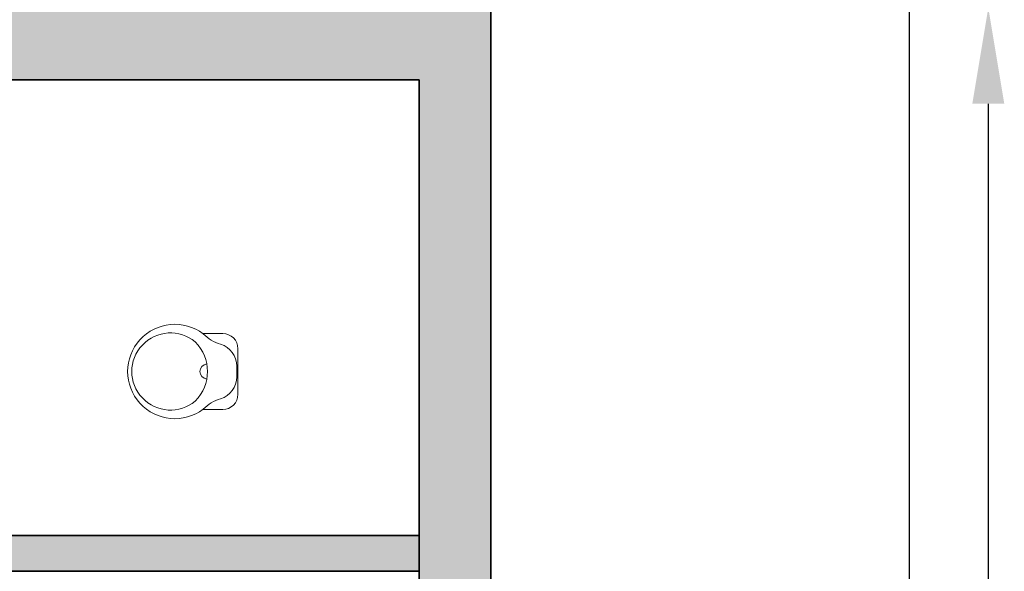
# Model space of a CAD drawing. Units: inches. Extents: x 2083 to 3317, y 1141 to 2115.
# Tile 249 of 256: x 3068 to 3191, y 1416 to 1485. Entities that reach past the tile are written whole.
import ezdxf

# ---------------------------------------------------------------- set-up
doc = ezdxf.new("R2010")
doc.units = ezdxf.units.IN
for name, color, linetype, lineweight in [('A-ANNO-DIMS', 2, 'Continuous', 18), ('A-FLOR-CASE', 8, 'Continuous', 18), ('A-FLOR-FIXT', 9, 'Continuous', 18), ('A-WALL', 7, 'Continuous', 35)]:
    doc.layers.add(name, color=color, linetype=linetype, lineweight=lineweight)
doc.layers.add('A-WALL-PATT', color=251, linetype='Continuous', lineweight=13, true_color=0x636466)
doc.styles.get("Standard").update_dxf_attribs({"font": 'arial.ttf'})
doc.dimstyles.new('ISO-25', dxfattribs={"dimtxt": 12, "dimasz": 12, "dimexe": 1.25, "dimexo": 0.625, "dimtad": 1, "dimlunit": 3, "dimtxsty": 'Standard', "dimcen": 2.5, "dimadec": 0, "dimazin": 0, "dimtfac": 1, "dimtmove": 0, "dimatfit": 3, "dimfxl": 1, "dimarcsym": 0})

# ---------------------------------------------------------------- blocks, each defined once
blk = doc.blocks.new('A$C6EF51710')
at = {"linetype": 'ByBlock'}
for p, q in [((0.0508, 0.2843), (0.1169, 0.2843)), ((0, 0.0811), (0, 0.2335)), ((0.0041, 0.1392), (0.0041, 0.1755)), ((0.1169, 0.0303), (0.0508, 0.0303))]:
    blk.add_line(p, q, dxfattribs=at)
for centre, radius, start, end in [((0.2107, 0.1573), 0.1576, 232.8984, 127.1016), ((0.0508, 0.2335), 0.0508, 90, 180), ((0.0168, 0.3818), 0.1397, 287.1046, 315), ((0.2254, 0.1573), 0.1289, 230.0084, 129.9916), ((0.0803, 0.1755), 0.0762, 107.1046, 180), ((0.2413, 0.1573), 0.1397, 135, 225), ((0.1016, 0.1573), 0.0254, 275.2159, 84.7841), ((0.0803, 0.1392), 0.0762, 180, 252.8954), ((0.0508, 0.0811), 0.0508, 180, 270), ((0.0168, -0.0672), 0.1397, 45, 72.8954)]:
    blk.add_arc(centre, radius, start, end, dxfattribs=at)
blk = doc.blocks.new('*D9')
at = {"layer": 'A-ANNO-DIMS', "color": 0, "lineweight": -2, "transparency": 16777216}
for p, q in [((3127.58, 1486.76), (3190.4, 1486.76)), ((3189.15, 1474.76), (3189.15, 1275.26)), ((3127.58, 1263.26), (3190.4, 1263.26))]:
    blk.add_line(p, q, dxfattribs=at)
at = {"layer": 'A-ANNO-DIMS', "color": 0, "transparency": 16777216}
for points in [[(3187.15, 1474.76), (3191.15, 1474.76), (3189.15, 1486.76)], [(3187.15, 1275.26), (3191.15, 1275.26), (3189.15, 1263.26)]]:
    blk.add_solid(points, dxfattribs=at)
at = {"layer": 'Defpoints', "color": 0, "transparency": 16777216}
for p in [(3126.96, 1486.76), (3126.96, 1263.26), (3189.15, 1263.26)]:
    blk.add_point(p, dxfattribs=at)
at = {"layer": 'A-ANNO-DIMS', "color": 0, "transparency": 16777216, "insert": (3182.4, 1375.01), "char_height": 12, "attachment_point": 5, "rotation": 90}
blk.add_mtext('18\'-7.5"', dxfattribs=at)
blk = doc.blocks.new('CASEWORK-96X24')
for q in [(0, 0), (24, 96)]:
    blk.add_line((0, 96), q)
blk = doc.blocks.new('*D35')
at = {"layer": 'A-ANNO-DIMS', "color": 0, "lineweight": -2, "transparency": 16777216}
for p, q in [((3127.58, 2020.76), (3180.56, 2020.76)), ((3179.31, 1275.26), (3179.31, 2008.76)), ((3127.58, 1263.26), (3180.56, 1263.26))]:
    blk.add_line(p, q, dxfattribs=at)
at = {"layer": 'A-ANNO-DIMS', "color": 0, "transparency": 16777216}
for points in [[(3177.31, 2008.76), (3181.31, 2008.76), (3179.31, 2020.76)], [(3177.31, 1275.26), (3181.31, 1275.26), (3179.31, 1263.26)]]:
    blk.add_solid(points, dxfattribs=at)
at = {"layer": 'Defpoints', "color": 0, "transparency": 16777216}
for p in [(3126.96, 2020.76), (3179.31, 2020.76), (3126.96, 1263.26)]:
    blk.add_point(p, dxfattribs=at)
at = {"layer": 'A-ANNO-DIMS', "color": 0, "transparency": 16777216, "insert": (3172.48, 1642.01), "char_height": 12, "attachment_point": 5, "rotation": 90}
blk.add_mtext('63\'-1 1/2"', dxfattribs=at)

msp = doc.modelspace()

# ---------------------------------------------------------------- hatches: boundary and pattern name
at = {"layer": 'A-WALL-PATT'}
h = msp.add_hatch(color=256, dxfattribs=at)
h.dxf.hatch_style = 1
h.paths.add_polyline_path([(3126.96, 2020.761), (2748.96, 2020.761), (2604.96, 2020.761), (2226.96, 2020.761), (2226.96, 1702.761), (2466.96, 1702.761), (2466.96, 1582.761), (2418.96, 1582.761), (2418.96, 1477.761), (2226.96, 1477.761), (2226.96, 1263.261), (2544.96, 1263.261), (2544.96, 1411.761), (2604.96, 1411.761), (2685.96, 1411.761), (2685.96, 1420.761), (2604.96, 1420.761), (2604.96, 1573.761), (2604.96, 1702.761), (2604.96, 2011.761), (2748.96, 2011.761), (2748.96, 1702.761), (2862.96, 1702.761), (2862.96, 1621.761), (2871.96, 1621.761), (2871.96, 1702.761), (2883.96, 1702.761), (2883.96, 1706.939, -0.0264593), (2883.96, 1711.761), (2757.96, 1711.761), (2757.96, 1807.761), (2787.96, 1807.761), (2787.96, 1812.261), (2757.96, 1812.261), (2757.96, 2011.761), (2877.96, 2011.761), (2877.96, 1812.261), (2847.96, 1812.261), (2847.96, 1807.761), (2889.836, 1807.761), (2889.836, 1812.261), (2882.46, 1812.261), (2882.46, 2011.761), (3117.96, 2011.761), (3117.96, 1812.261), (2937.836, 1812.261), (2937.836, 1807.761), (2995.71, 1807.761), (2995.71, 1796.118), (3000.21, 1796.118), (3000.21, 1807.761), (3117.96, 1807.761), (3117.96, 1711.761), (3000.21, 1711.761), (3000.21, 1760.118), (2998.573, 1760.118, -0.020711), (2995.71, 1760.118), (2995.71, 1711.761), (2931.96, 1711.761), (2931.96, 1702.761), (3126.96, 1702.761)])
h.paths.add_polyline_path([(2471.46, 2011.761), (2471.46, 1810.011), (2462.717, 1810.011), (2462.717, 1805.511), (2505.96, 1805.511), (2505.96, 1810.011), (2475.96, 1810.011), (2475.96, 2011.761), (2595.96, 2011.761), (2595.96, 1810.011), (2565.96, 1810.011), (2565.96, 1805.511), (2595.96, 1805.511), (2595.96, 1711.761), (2235.96, 1711.761), (2235.96, 1805.511), (2353.71, 1805.511), (2353.71, 1796.054), (2358.21, 1796.054), (2358.21, 1805.511), (2414.717, 1805.511), (2414.717, 1810.011), (2235.96, 1810.011), (2235.96, 2011.761)], flags=16)
h.paths.add_polyline_path([(2270.205, 1994.61), (2270.205, 1970.61), (2246.205, 1970.61), (2246.205, 1994.61)], flags=0)
edge = h.paths.add_edge_path(flags=0)
edge.add_ellipse((2332.027, 1899.798), major_axis=(-3.043, 3.043), ratio=0.1682525, start_angle=-161.33217, end_angle=-156.30711, ccw=False)
edge.add_ellipse((2333.082, 1898.744), major_axis=(-1.055, 1.055), ratio=0.4535321, start_angle=-123.37102, end_angle=-94.15911)
edge = h.paths.add_edge_path(flags=0)
edge.add_ellipse((2332.027, 1968.876), major_axis=(3.043, 3.043), ratio=0.1682525, start_angle=18.66783, end_angle=23.69289)
edge.add_spline(control_points=[(2332.926, 1970.691), (2332.227, 1970.336), (2330.894, 1969.659), (2328.413, 1970.932), (2327.204, 1967.749), (2324.71, 1969.956), (2322.533, 1967.012), (2320.013, 1971.296), (2317.68, 1968.158), (2316.041, 1967.102), (2315.427, 1966.81)], knot_values=[0, 0, 0, 0, 2.2670587, 4.3245589, 6.6855835, 8.8786411, 11.121502, 14.300359, 17.7552837, 19.732645, 19.732645, 19.732645, 19.732645], degree=3, periodic=0)
edge.add_ellipse((2332.027, 1968.876), major_axis=(3.043, 3.043), ratio=0.1682525, start_angle=18.66783, end_angle=23.69289, ccw=False)
edge.add_ellipse((2333.082, 1969.931), major_axis=(1.055, 1.055), ratio=0.4535321, start_angle=56.62898, end_angle=85.84089, ccw=False)
edge = h.paths.add_edge_path(flags=0)
edge.add_spline(control_points=[(2296.428, 1967.988), (2293.628, 1965.336), (2287.704, 1959.727), (2299.744, 1949.996), (2294.533, 1935.669), (2290.573, 1920.604), (2293.394, 1909.974), (2296.185, 1904.967)], knot_values=[0.0991853, 0.0991853, 0.0991853, 0.0991853, 0.3453009, 0.6198217, 0.9826526, 1.3860932, 1.8105546, 1.8105546, 1.8105546, 1.8105546], degree=3, periodic=0)
edge.add_spline(control_points=[(2296.185, 1904.967), (2297.384, 1902.619), (2298.001, 1901.949), (2298.553, 1901.468)], knot_values=[0.0062457, 0.0062457, 0.0062457, 0.0062457, 0.0554759, 0.0554759, 0.0554759, 0.0554759], degree=3, periodic=0)
edge.add_spline(control_points=[(2298.553, 1901.468), (2297.259, 1900.923), (2295.225, 1900.232), (2293.06, 1900.614), (2292.101, 1900.788), (2292.09, 1900.791)], knot_values=[0.3128349, 0.3128349, 0.3128349, 0.3128349, 0.4017797, 0.4749867, 0.4759027, 0.4759027, 0.4759027, 0.4759027], degree=3, periodic=0)
edge.add_arc((2292.794, 1904.664), 3.937, 215.4209, 259.69818, ccw=False)
edge.add_spline(control_points=[(2289.585, 1902.382), (2289.477, 1902.535), (2289.368, 1902.688), (2289.261, 1902.841)], knot_values=[0.1028719, 0.1028719, 0.1028719, 0.1028719, 0.1168958, 0.1168958, 0.1168958, 0.1168958], degree=3, periodic=0)
edge.add_spline(control_points=[(2289.261, 1902.841), (2288.687, 1902.55), (2287.64, 1902.02), (2285.881, 1901.874), (2283.853, 1901.504), (2281.72, 1899.711), (2278.467, 1899.493), (2276.157, 1901.883), (2272.259, 1899.804), (2267.778, 1901.843), (2262.244, 1900.184), (2257.415, 1901.782), (2254.318, 1900.726), (2253.178, 1900.337)], knot_values=[0, 0, 0, 0, 1.9079767, 3.4771759, 5.261074, 7.9728515, 11.6802485, 13.7179214, 16.9395917, 22.789562, 27.5025027, 33.5952153, 37.1456181, 37.1456181, 37.1456181, 37.1456181], degree=3, periodic=0)
edge.add_line((2253.178, 1900.337), (2250.244, 1902.841))
edge.add_line((2250.244, 1902.841), (2250.244, 1965.833))
edge.add_line((2250.244, 1965.833), (2253.178, 1968.337))
edge.add_spline(control_points=[(2253.178, 1968.337), (2254.318, 1967.948), (2257.415, 1966.892), (2262.244, 1968.49), (2267.778, 1966.831), (2271.527, 1968.537), (2273.876, 1967.828), (2274.207, 1967.728)], knot_values=[0, 0, 0, 0, 0.0901802, 0.2449351, 0.3646438, 0.5132331, 0.5378548, 0.5378548, 0.5378548, 0.5378548], degree=3, periodic=0)
edge.add_arc((2274.353, 1963.793), 3.937, 72.05113, 92.12795, ccw=False)
edge.add_arc((2281.297, 1985.23), 18.596, 252.05113, 288.56572)
edge.add_arc((2292.317, 1956.029), 12.646, 71.02679, 113.77822, ccw=False)
edge = h.paths.add_edge_path(flags=0)
edge.add_spline(control_points=[(2274.899, 1951.856), (2275.066, 1951.617), (2275.233, 1951.377), (2275.398, 1951.136)], knot_values=[1.4099157, 1.4099157, 1.4099157, 1.4099157, 1.4315903, 1.4315903, 1.4315903, 1.4315903], degree=3, periodic=0)
edge.add_spline(control_points=[(2275.398, 1951.136), (2275.792, 1950.562), (2276.179, 1949.984), (2276.546, 1949.397)], knot_values=[1.3582378, 1.3582378, 1.3582378, 1.3582378, 1.4099157, 1.4099157, 1.4099157, 1.4099157], degree=3, periodic=0)
edge.add_line((2276.546, 1949.397), (2277.437, 1947.862))
edge.add_spline(control_points=[(2277.437, 1947.862), (2276.304, 1945.673), (2274.64, 1942.427), (2274.632, 1938.094), (2272.799, 1930.852), (2274.356, 1943.897), (2275.948, 1947.923), (2276.546, 1949.397)], knot_values=[0.0056315, 0.0056315, 0.0056315, 0.0056315, 0.1860139, 0.2660015, 0.3570872, 0.5963902, 0.7397317, 0.7397317, 0.7397317, 0.7397317], degree=3, periodic=0)
edge.add_spline(control_points=[(2276.546, 1949.397), (2276.179, 1949.984), (2275.792, 1950.562), (2275.398, 1951.136)], knot_values=[1.3582378, 1.3582378, 1.3582378, 1.3582378, 1.4099157, 1.4099157, 1.4099157, 1.4099157], degree=3, periodic=0)
edge.add_spline(control_points=[(2275.398, 1951.136), (2274.943, 1950.08), (2274.208, 1948.025), (2273.935, 1944.851), (2272.469, 1937.627), (2273.466, 1945.696), (2274.701, 1951.059), (2274.899, 1951.856)], knot_values=[0.1043639, 0.1043639, 0.1043639, 0.1043639, 0.1896363, 0.2696239, 0.3607096, 0.6000126, 0.6446217, 0.6446217, 0.6446217, 0.6446217], degree=3, periodic=0)
h.paths.add_polyline_path([(2269.168, 1963.128, -0.3575267), (2268.171, 1960.976, -0.0925607), (2268.171, 1939.436, -0.3575267), (2269.168, 1937.285, -0.3575267), (2267.016, 1938.282, -0.1647847), (2254.686, 1938.282, -0.3575267), (2252.534, 1937.285, -0.3575267), (2253.531, 1939.436, -0.0925607), (2253.531, 1960.976, -0.3575267), (2252.534, 1963.128, -0.3575267), (2254.686, 1962.131, -0.1647847), (2267.016, 1962.131, -0.3575267)], flags=0)
h.paths.add_polyline_path([(2248.874, 1967.802), (2248.874, 1957.028), (2249.458, 1957.028), (2249.458, 1911.647), (2248.874, 1911.647), (2248.874, 1900.873), (2246.512, 1900.873, 0.1973271), (2244.15, 1902.457), (2244.15, 1966.218, 0.1973271), (2246.512, 1967.802)], flags=0)
h.paths.add_polyline_path([(2269.168, 1931.389, -0.3575267), (2268.171, 1929.238, -0.0925607), (2268.171, 1907.698, -0.3575267), (2269.168, 1905.547, -0.3575267), (2267.016, 1906.544, -0.1647847), (2254.686, 1906.544, -0.3575267), (2252.534, 1905.547, -0.3575267), (2253.531, 1907.698, -0.0925607), (2253.531, 1929.238, -0.3575267), (2252.534, 1931.389, -0.3575267), (2254.686, 1930.392, -0.1647847), (2267.016, 1930.392, -0.3575267)], flags=0)
edge = h.paths.add_edge_path(flags=0)
edge.add_spline(control_points=[(2276.197, 1906.724), (2276.168, 1909.029), (2276.114, 1913.372), (2270.598, 1924.925), (2273.905, 1919.013), (2275.922, 1916.262), (2275.475, 1912.402), (2277.258, 1910.381), (2276.696, 1908.225), (2276.646, 1906.813), (2276.618, 1906.008)], knot_values=[0, 0, 0, 0, 8.6102597, 16.2212739, 18.8430575, 23.8048978, 27.4408283, 29.3561016, 31.2034776, 33.6506866, 33.6506866, 33.6506866, 33.6506866], degree=3, periodic=0)
edge.add_spline(control_points=[(2276.618, 1906.008), (2276.623, 1905.624), (2276.498, 1904.629), (2275.442, 1903.855), (2274.937, 1903.08), (2274.859, 1902.841)], knot_values=[0.1564884, 0.1564884, 0.1564884, 0.1564884, 0.1843975, 0.2313765, 0.2505985, 0.2505985, 0.2505985, 0.2505985], degree=3, periodic=0)
edge.add_line((2274.859, 1902.841), (2276.506, 1902.841))
edge.add_spline(control_points=[(2276.506, 1902.841), (2276.788, 1903.085), (2277.665, 1904.125), (2278.25, 1904.341), (2277.654, 1908.527), (2278.156, 1906.228), (2278.1, 1905.286), (2278.847, 1904.069), (2277.857, 1903.415), (2277.874, 1902.991), (2277.904, 1902.841)], knot_values=[0.0595743, 0.0595743, 0.0595743, 0.0595743, 0.0807529, 0.1037415, 0.1697201, 0.1760361, 0.2071372, 0.2404744, 0.2623409, 0.2736605, 0.2736605, 0.2736605, 0.2736605], degree=3, periodic=0)
edge.add_line((2277.904, 1902.841), (2280.03, 1902.841))
edge.add_spline(control_points=[(2280.03, 1902.841), (2279.888, 1903.088), (2279.499, 1903.982), (2280.152, 1905.939), (2278.104, 1909.658), (2279.762, 1907.185), (2280.328, 1904.875), (2280.485, 1903.49), (2281.463, 1903.249), (2281.758, 1902.936), (2281.834, 1902.841)], knot_values=[0.013856, 0.013856, 0.013856, 0.013856, 0.0348738, 0.0888667, 0.1078792, 0.1267378, 0.158714, 0.1937575, 0.2174868, 0.2267221, 0.2267221, 0.2267221, 0.2267221], degree=3, periodic=0)
edge.add_spline(control_points=[(2281.834, 1902.841), (2281.788, 1902.827), (2281.647, 1902.783), (2281.396, 1902.859), (2281.088, 1902.985), (2280.721, 1903.061), (2280.333, 1903.026), (2280.125, 1902.899), (2280.03, 1902.841)], knot_values=[0, 0, 0, 0, 0.1441304, 0.435517, 0.7492759, 1.1530457, 1.5483707, 1.878348, 1.878348, 1.878348, 1.878348], degree=3, periodic=0)
edge.add_line((2280.03, 1902.841), (2277.904, 1902.841))
edge.add_spline(control_points=[(2277.904, 1902.841), (2277.893, 1902.796), (2277.865, 1902.68), (2277.607, 1902.687), (2277.274, 1902.801), (2276.838, 1902.62), (2276.584, 1902.789), (2276.506, 1902.841)], knot_values=[0, 0, 0, 0, 0.1271885, 0.3261988, 0.6280094, 1.2435704, 1.5153306, 1.5153306, 1.5153306, 1.5153306], degree=3, periodic=0)
edge.add_line((2276.506, 1902.841), (2274.859, 1902.841))
edge.add_spline(control_points=[(2274.859, 1902.841), (2274.814, 1902.899), (2274.725, 1903.013), (2274.493, 1903.119), (2274.244, 1902.961), (2273.937, 1903.185), (2273.614, 1902.983), (2273.408, 1902.883), (2273.322, 1902.841)], knot_values=[0, 0, 0, 0, 0.2184302, 0.4369566, 0.6879766, 0.9903786, 1.3983955, 1.6918498, 1.6918498, 1.6918498, 1.6918498], degree=3, periodic=0)
edge.add_spline(control_points=[(2273.322, 1902.841), (2273.617, 1903.446), (2274.274, 1904.538), (2276.027, 1904.574), (2276.207, 1906.584), (2276.197, 1906.724)], knot_values=[0.0122268, 0.0122268, 0.0122268, 0.0122268, 0.0594721, 0.1062177, 0.134458, 0.134458, 0.134458, 0.134458], degree=3, periodic=0)
h.paths.add_polyline_path([(2270.776, 1897.79), (2270.776, 1873.79), (2246.776, 1873.79), (2246.776, 1897.79)], flags=0)
h.paths.add_polyline_path([(2353.71, 1760.005), (2353.71, 1760.054), (2358.21, 1760.054, -0.033729)], flags=0)
h.paths.add_polyline_path([(2321.819, 1737.529), (2341.995, 1737.529, -0.4142136), (2343.203, 1736.321), (2343.203, 1721.021, -0.4142136), (2341.995, 1719.813), (2321.819, 1719.813, -0.4142136), (2320.611, 1721.021), (2320.611, 1736.321, -0.4142136)], flags=0)
h.paths.add_polyline_path([(2324.235, 1736.321), (2339.579, 1736.321, -0.4142136), (2341.995, 1733.905), (2341.995, 1725.45, -0.4142136), (2339.579, 1723.034), (2333.681, 1723.034), (2333.845, 1722.045, -0.8706461), (2335.425, 1721.826, -0.767327), (2333.923, 1721.423), (2331.291, 1721.423, -0.767327), (2329.788, 1721.826, -0.8706461), (2331.368, 1722.045), (2331.533, 1723.034), (2324.235, 1723.034, -0.4142136), (2321.819, 1725.45), (2321.819, 1733.905, -0.4142136)], flags=0)
h.paths.add_polyline_path([(2570.484, 1928.615), (2589.684, 1928.615), (2590.169, 1928.615), (2590.169, 1904.993), (2570.484, 1904.993)], flags=0)
h.paths.add_polyline_path([(2574.447, 1927.264, -1), (2572.829, 1927.264, -1)], flags=0)
h.paths.add_polyline_path([(2573.09, 1926.941), (2573.925, 1927.776), (2574.148, 1927.553), (2573.313, 1926.718)], flags=0)
h.paths.add_polyline_path([(2578.779, 1919.73, -1), (2571.592, 1919.73, -1)], flags=0)
h.paths.add_polyline_path([(2578.385, 1919.73, -1), (2571.985, 1919.73, -1)], flags=0)
h.paths.add_polyline_path([(2331.596, 1729.476, -1), (2333.618, 1729.476, -1)], flags=0)
h.paths.add_polyline_path([(2578.034, 1927.264, -1), (2576.416, 1927.264, -1)], flags=0)
h.paths.add_polyline_path([(2576.689, 1927.531), (2576.912, 1927.754), (2577.747, 1926.919), (2577.524, 1926.696)], flags=0)
h.paths.add_polyline_path([(2578.139, 1909.86, -1), (2572.232, 1909.86, -1)], flags=0)
h.paths.add_polyline_path([(2577.745, 1909.86, -1), (2572.625, 1909.86, -1)], flags=0)
h.paths.add_polyline_path([(2583.798, 1927.264, -1), (2582.179, 1927.264, -1)], flags=0)
h.paths.add_polyline_path([(2582.719, 1927.754), (2583.554, 1926.919), (2583.331, 1926.696), (2582.496, 1927.531)], flags=0)
h.paths.add_polyline_path([(2582.496, 1927.531), (2582.719, 1927.754), (2583.554, 1926.919), (2583.331, 1926.696)], flags=0)
h.paths.add_polyline_path([(2587.739, 1920.53, -1), (2581.832, 1920.53, -1)], flags=0)
h.paths.add_polyline_path([(2587.345, 1920.53, -1), (2582.225, 1920.53, -1)], flags=0)
h.paths.add_polyline_path([(2587.385, 1927.264, -1), (2585.766, 1927.264, -1)], flags=0)
h.paths.add_polyline_path([(2586.082, 1926.98), (2586.917, 1927.815), (2587.14, 1927.593), (2586.305, 1926.758)], flags=0)
h.paths.add_polyline_path([(2588.379, 1910.66, -1), (2581.192, 1910.66, -1)], flags=0)
h.paths.add_polyline_path([(2587.985, 1910.66, -1), (2581.585, 1910.66, -1)], flags=0)
h.paths.add_polyline_path([(2417.168, 1729.478), (2437.344, 1729.478, -0.4142136), (2438.552, 1728.27), (2438.552, 1712.969, -0.4142136), (2437.344, 1711.761), (2417.168, 1711.761, -0.4142136), (2415.96, 1712.969), (2415.96, 1728.27, -0.4142136)], flags=0)
h.paths.add_polyline_path([(2419.584, 1728.27), (2434.928, 1728.27, -0.4142136), (2437.344, 1725.854), (2437.344, 1717.398, -0.4142136), (2434.928, 1714.983), (2429.029, 1714.983), (2429.194, 1713.994, -0.8706461), (2430.774, 1713.775, -0.767327), (2429.271, 1713.372), (2426.64, 1713.372, -0.767327), (2425.137, 1713.775, -0.8706461), (2426.717, 1713.994), (2426.882, 1714.983), (2419.584, 1714.983, -0.4142136), (2417.168, 1717.398), (2417.168, 1725.854, -0.4142136)], flags=0)
h.paths.add_polyline_path([(2419.584, 1728.27), (2434.928, 1728.27, -0.4142136), (2437.344, 1725.854), (2437.344, 1717.398, -0.4142136), (2434.928, 1714.983), (2429.029, 1714.983), (2428.358, 1719.009), (2427.553, 1719.009), (2426.882, 1714.983), (2419.584, 1714.983, -0.4142136), (2417.168, 1717.398), (2417.168, 1725.854, -0.4142136)], flags=0)
h.paths.add_polyline_path([(2426.944, 1721.425, -1), (2428.967, 1721.425, -1)], flags=0)
h.paths.add_polyline_path([(2475.96, 1702.761), (2595.96, 1702.761), (2595.96, 1582.761), (2475.96, 1582.761)], flags=16)
h.paths.add_polyline_path([(2427.96, 1573.761), (2595.96, 1573.761), (2595.96, 1468.761), (2595.96, 1420.761), (2384.46, 1420.761), (2384.46, 1468.761), (2427.96, 1468.761)], flags=16)
h.paths.add_polyline_path([(2379.96, 1468.761), (2379.96, 1420.761), (2235.96, 1420.761), (2235.96, 1468.761)], flags=16)
h.paths.add_polyline_path([(2317.816, 1466.696), (2337.992, 1466.696, -0.4142136), (2339.2, 1465.488), (2339.2, 1450.187, -0.4142136), (2337.992, 1448.979), (2317.816, 1448.979, -0.4142136), (2316.608, 1450.187), (2316.608, 1465.488, -0.4142136)], flags=0)
h.paths.add_polyline_path([(2320.232, 1465.488), (2335.576, 1465.488, -0.4142136), (2337.992, 1463.072), (2337.992, 1454.616, -0.4142136), (2335.576, 1452.2), (2329.677, 1452.2), (2329.842, 1451.212, -0.8706461), (2331.422, 1450.992, -0.767327), (2329.92, 1450.59), (2327.288, 1450.59, -0.767327), (2325.785, 1450.992, -0.8706461), (2327.365, 1451.212), (2327.53, 1452.2), (2320.232, 1452.2, -0.4142136), (2317.816, 1454.616), (2317.816, 1463.072, -0.4142136)], flags=0)
h.paths.add_polyline_path([(2320.232, 1465.488), (2335.576, 1465.488, -0.4142136), (2337.992, 1463.072), (2337.992, 1454.616, -0.4142136), (2335.576, 1452.2), (2329.677, 1452.2), (2329.006, 1456.227), (2328.201, 1456.227), (2327.53, 1452.2), (2320.232, 1452.2, -0.4142136), (2317.816, 1454.616), (2317.816, 1463.072, -0.4142136)], flags=0)
h.paths.add_polyline_path([(2327.593, 1458.643, -1), (2329.615, 1458.643, -1)], flags=0)
h.paths.add_polyline_path([(2244.412, 1433.34), (2241.921, 1433.34, -0.4142136), (2240.018, 1435.244), (2240.018, 1440.953, -0.4142105), (2241.921, 1442.856), (2244.412, 1442.856, -1.9764724)], flags=0)
h.paths.add_polyline_path([(2245.357, 1434.398, -0.4142136), (2245.357, 1441.799, -2.1440985)], flags=0)
h.paths.add_polyline_path([(2535.96, 1416.261), (2535.96, 1272.261), (2235.96, 1272.261), (2235.96, 1416.261)], flags=16)
h.paths.add_polyline_path([(2260.12, 1384.293), (2260.12, 1362.039), (2237.865, 1362.039), (2237.865, 1384.293)], flags=0)
edge = h.paths.add_edge_path(flags=0)
edge.add_line((2318.252, 1362.093), (2318.146, 1362.001))
edge.add_ellipse((2317.445, 1360.431), major_axis=(2.822, 2.822), ratio=0.1682525, start_angle=18.66783, end_angle=20.94813, ccw=False)
edge.add_ellipse((2318.423, 1361.409), major_axis=(0.978, 0.978), ratio=0.4535321, start_angle=56.62898, end_angle=70.2262, ccw=False)
edge = h.paths.add_edge_path(flags=0)
edge.add_line((2319.107, 1295.571), (2319.015, 1295.677))
edge.add_ellipse((2317.445, 1296.378), major_axis=(-2.822, 2.822), ratio=0.1682525, start_angle=-161.33217, end_angle=-159.05187, ccw=False)
edge.add_ellipse((2318.423, 1295.4), major_axis=(-0.978, 0.978), ratio=0.4535321, start_angle=-123.37102, end_angle=-109.7738)
edge = h.paths.add_edge_path(flags=0)
edge.add_spline(control_points=[(2284.21, 1301.17), (2284.581, 1300.445), (2284.891, 1299.892), (2285.16, 1299.461)], knot_values=[0.0390658, 0.0390658, 0.0390658, 0.0390658, 0.0554759, 0.0554759, 0.0554759, 0.0554759], degree=3, periodic=0)
edge.add_line((2285.16, 1299.461), (2284.21, 1301.17))
edge = h.paths.add_edge_path(flags=0)
edge.add_line((2280.412, 1297.298), (2283.37, 1297.036))
edge.add_line((2283.37, 1297.036), (2286.406, 1297.926))
edge.add_spline(control_points=[(2286.406, 1297.926), (2285.305, 1297.463), (2284.345, 1297.129), (2283.37, 1297.036)], knot_values=[0.3943688, 0.3943688, 0.3943688, 0.3943688, 0.4759027, 0.4759027, 0.4759027, 0.4759027], degree=3, periodic=0)
edge.add_spline(control_points=[(2283.37, 1297.036), (2283.281, 1297.028), (2282.316, 1296.957), (2281.313, 1297.134), (2280.423, 1297.296), (2280.412, 1297.298)], knot_values=[0.3128349, 0.3128349, 0.3128349, 0.3128349, 0.3202458, 0.3934528, 0.3943688, 0.3943688, 0.3943688, 0.3943688], degree=3, periodic=0)
edge = h.paths.add_edge_path(flags=0)
edge.add_line((2284.436, 1359.607), (2280.446, 1355.328))
edge.add_line((2280.446, 1355.328), (2279.58, 1351.018))
edge.add_line((2279.58, 1351.018), (2282.413, 1346.58))
edge.add_spline(control_points=[(2282.413, 1346.58), (2283.153, 1345.589), (2284.253, 1344.029), (2284.801, 1342.387), (2284.935, 1341.806)], knot_values=[1.2400982, 1.2400982, 1.2400982, 1.2400982, 1.3328922, 1.3827123, 1.3827123, 1.3827123, 1.3827123], degree=3, periodic=0)
edge.add_spline(control_points=[(2284.935, 1341.806), (2285.319, 1340.141), (2285.233, 1338.409), (2284.91, 1336.654)], knot_values=[1.0974841, 1.0974841, 1.0974841, 1.0974841, 1.2400982, 1.2400982, 1.2400982, 1.2400982], degree=3, periodic=0)
edge.add_spline(control_points=[(2284.91, 1336.654), (2284.587, 1334.899), (2284.027, 1333.12), (2283.463, 1331.361)], knot_values=[0.9548699, 0.9548699, 0.9548699, 0.9548699, 1.0974841, 1.0974841, 1.0974841, 1.0974841], degree=3, periodic=0)
edge.add_line((2283.463, 1331.361), (2281.89, 1326.153))
edge.add_line((2281.89, 1326.153), (2280.756, 1321.056))
edge.add_line((2280.756, 1321.056), (2280.299, 1316.002))
edge.add_line((2280.299, 1316.002), (2280.716, 1310.95))
edge.add_line((2280.716, 1310.95), (2282.028, 1305.972))
edge.add_line((2282.028, 1305.972), (2284.21, 1301.17))
edge.add_spline(control_points=[(2284.21, 1301.17), (2283.341, 1302.73), (2282.612, 1304.336), (2282.028, 1305.972)], knot_values=[0.0991853, 0.0991853, 0.0991853, 0.0991853, 0.2417994, 0.2417994, 0.2417994, 0.2417994], degree=3, periodic=0)
edge.add_spline(control_points=[(2282.028, 1305.972), (2281.444, 1307.608), (2281.005, 1309.273), (2280.716, 1310.95)], knot_values=[0.2417994, 0.2417994, 0.2417994, 0.2417994, 0.3844135, 0.3844135, 0.3844135, 0.3844135], degree=3, periodic=0)
edge.add_spline(control_points=[(2280.716, 1310.95), (2280.433, 1312.588), (2280.289, 1314.277), (2280.299, 1315.962), (2280.299, 1316.002)], knot_values=[0.3844135, 0.3844135, 0.3844135, 0.3844135, 0.5236467, 0.5270276, 0.5270276, 0.5270276, 0.5270276], degree=3, periodic=0)
edge.add_spline(control_points=[(2280.299, 1316.002), (2280.312, 1317.687), (2280.478, 1319.368), (2280.756, 1321.056)], knot_values=[0.5270276, 0.5270276, 0.5270276, 0.5270276, 0.6696417, 0.6696417, 0.6696417, 0.6696417], degree=3, periodic=0)
edge.add_spline(control_points=[(2280.756, 1321.056), (2281.035, 1322.744), (2281.426, 1324.44), (2281.89, 1326.153)], knot_values=[0.6696417, 0.6696417, 0.6696417, 0.6696417, 0.8122558, 0.8122558, 0.8122558, 0.8122558], degree=3, periodic=0)
edge.add_spline(control_points=[(2281.89, 1326.153), (2282.264, 1327.533), (2282.788, 1329.262), (2283.353, 1331.018), (2283.463, 1331.361)], knot_values=[0.8122558, 0.8122558, 0.8122558, 0.8122558, 0.9270873, 0.9548699, 0.9548699, 0.9548699, 0.9548699], degree=3, periodic=0)
edge.add_line((2283.463, 1331.361), (2284.91, 1336.654))
edge.add_line((2284.91, 1336.654), (2284.935, 1341.806))
edge.add_line((2284.935, 1341.806), (2282.413, 1346.58))
edge.add_spline(control_points=[(2282.413, 1346.58), (2281.275, 1348.104), (2280.078, 1349.57), (2279.58, 1351.018)], knot_values=[1.3827123, 1.3827123, 1.3827123, 1.3827123, 1.5253264, 1.5253264, 1.5253264, 1.5253264], degree=3, periodic=0)
edge.add_spline(control_points=[(2279.58, 1351.018), (2279.443, 1351.415), (2279.136, 1352.857), (2279.735, 1354.29), (2280.446, 1355.328)], knot_values=[1.5253264, 1.5253264, 1.5253264, 1.5253264, 1.564439, 1.6679405, 1.6679405, 1.6679405, 1.6679405], degree=3, periodic=0)
edge.add_spline(control_points=[(2280.446, 1355.328), (2281.426, 1356.758), (2282.931, 1358.183), (2284.436, 1359.607)], knot_values=[1.6679405, 1.6679405, 1.6679405, 1.6679405, 1.8105546, 1.8105546, 1.8105546, 1.8105546], degree=3, periodic=0)
edge.add_arc((2280.623, 1348.518), 11.726, 71.02679, 113.77822)
edge.add_arc((2270.405, 1375.595), 17.244, 252.05113, 288.56572, ccw=False)
edge.add_arc((2263.966, 1355.718), 3.651, 72.05113, 92.12795)
edge.add_arc((2263.966, 1355.718), 3.651, 92.12795, 177.98513)
edge.add_spline(control_points=[(2260.318, 1355.846), (2260.26, 1354.221), (2260.551, 1350.187), (2262.999, 1346.766), (2264.473, 1344.649)], knot_values=[1.4315903, 1.4315903, 1.4315903, 1.4315903, 1.5641438, 1.7706953, 1.7706953, 1.7706953, 1.7706953], degree=3, periodic=0)
edge.add_line((2264.473, 1344.649), (2264.936, 1343.983))
edge.add_spline(control_points=[(2263.801, 1340.248), (2263.843, 1340.514), (2264.067, 1341.756), (2264.513, 1343.002), (2264.935, 1343.981)], knot_values=[0.5365702, 0.5365702, 0.5365702, 0.5365702, 0.5593494, 0.6446217, 0.6446217, 0.6446217, 0.6446217], degree=3, periodic=0)
edge.add_spline(control_points=[(2264.935, 1343.981), (2265.118, 1343.715), (2265.299, 1343.448), (2265.477, 1343.179)], knot_values=[1.3840767, 1.3840767, 1.3840767, 1.3840767, 1.4099157, 1.4099157, 1.4099157, 1.4099157], degree=3, periodic=0)
edge.add_spline(control_points=[(2265.477, 1343.179), (2265.655, 1342.911), (2265.829, 1342.641), (2265.999, 1342.369)], knot_values=[1.3582378, 1.3582378, 1.3582378, 1.3582378, 1.3840767, 1.3840767, 1.3840767, 1.3840767], degree=3, periodic=0)
edge.add_line((2265.999, 1342.369), (2266.826, 1340.946))
edge.add_spline(control_points=[(2266.826, 1340.946), (2268.894, 1337.09), (2271.398, 1325.843), (2270.516, 1310.569), (2275.919, 1301.861), (2277.79, 1299.199)], knot_values=[0.1168958, 0.1168958, 0.1168958, 0.1168958, 0.4729873, 1.0509689, 1.3137934, 1.3137934, 1.3137934, 1.3137934], degree=3, periodic=0)
edge.add_spline(control_points=[(2277.79, 1299.199), (2277.839, 1299.128), (2277.889, 1299.057), (2277.94, 1298.987)], knot_values=[0.1098839, 0.1098839, 0.1098839, 0.1098839, 0.1168958, 0.1168958, 0.1168958, 0.1168958], degree=3, periodic=0)
edge.add_line((2277.94, 1298.987), (2277.789, 1299.199))
edge.add_spline(control_points=[(2277.789, 1299.199), (2277.257, 1298.929), (2276.286, 1298.438), (2275.039, 1298.334), (2274.383, 1298.239), (2274.215, 1298.209)], knot_values=[33.1218702, 33.1218702, 33.1218702, 33.1218702, 35.0290557, 36.5982549, 37.1448269, 37.1448269, 37.1448269, 37.1448269], degree=3, periodic=0)
edge.add_line((2274.215, 1298.209), (2273.073, 1297.893))
edge.add_spline(control_points=[(2273.073, 1297.893), (2272.323, 1297.58), (2271.039, 1296.511), (2269.248, 1296.226), (2268.423, 1296.375)], knot_values=[26.5325843, 26.5325843, 26.5325843, 26.5325843, 29.198919, 31.8391012, 31.8391012, 31.8391012, 31.8391012], degree=3, periodic=0)
edge.add_line((2268.423, 1296.375), (2263.879, 1297.458))
edge.add_spline(control_points=[(2263.879, 1297.458), (2263.556, 1297.359), (2261.86, 1296.839), (2260.239, 1297.282), (2258.933, 1297.516)], knot_values=[15.9195506, 15.9195506, 15.9195506, 15.9195506, 16.9395917, 21.2260675, 21.2260675, 21.2260675, 21.2260675], degree=3, periodic=0)
edge.add_line((2258.933, 1297.516), (2254.055, 1297.329))
edge.add_spline(control_points=[(2254.055, 1297.329), (2253.756, 1297.296), (2252.114, 1297.165), (2250.462, 1297.544), (2249.13, 1297.668)], knot_values=[5.3065169, 5.3065169, 5.3065169, 5.3065169, 6.2764352, 10.6130337, 10.6130337, 10.6130337, 10.6130337], degree=3, periodic=0)
edge.add_line((2249.13, 1297.668), (2244.332, 1296.878))
edge.add_line((2244.332, 1296.878), (2241.611, 1299.199))
edge.add_line((2241.611, 1299.199), (2241.611, 1357.609))
edge.add_line((2241.611, 1357.609), (2244.332, 1359.931))
edge.add_line((2244.332, 1359.931), (2252.729, 1359.543))
edge.add_spline(control_points=[(2252.729, 1359.543), (2252.871, 1359.546), (2253.306, 1359.548), (2253.74, 1359.514), (2254.032, 1359.482)], knot_values=[0.233291, 0.233291, 0.233291, 0.233291, 0.2449351, 0.2689274, 0.2689274, 0.2689274, 0.2689274], degree=3, periodic=0)
edge.add_line((2254.032, 1359.482), (2259.587, 1359.416))
edge.add_spline(control_points=[(2259.587, 1359.416), (2260.677, 1359.629), (2262.073, 1359.897), (2263.524, 1359.459), (2263.83, 1359.366)], knot_values=[0.4225164, 0.4225164, 0.4225164, 0.4225164, 0.5132331, 0.5378548, 0.5378548, 0.5378548, 0.5378548], degree=3, periodic=0)
edge.add_arc((2263.966, 1355.718), 3.651, 72.05113, 92.12795, ccw=False)
edge.add_arc((2270.405, 1375.595), 17.244, 252.05113, 288.56572)
edge.add_arc((2280.623, 1348.518), 11.726, 71.02679, 113.77822, ccw=False)
h.paths.add_polyline_path([(2240.341, 1359.435), (2240.341, 1349.444), (2240.882, 1349.444), (2240.882, 1307.365), (2240.341, 1307.365), (2240.341, 1297.374), (2238.15, 1297.374, 0.1973271), (2235.96, 1298.843), (2235.96, 1357.966, 0.1973271), (2238.15, 1359.435)], flags=0)
h.paths.add_polyline_path([(2259.158, 1355.101, -0.3575267), (2258.233, 1353.106, -0.0925607), (2258.233, 1333.133, -0.3575267), (2259.158, 1331.138, -0.3575267), (2257.163, 1332.062, -0.1647847), (2245.729, 1332.062, -0.3575267), (2243.735, 1331.138, -0.3575267), (2244.659, 1333.133, -0.0925607), (2244.659, 1353.106, -0.3575267), (2243.735, 1355.101, -0.3575267), (2245.729, 1354.176, -0.1647847), (2257.163, 1354.176, -0.3575267)], flags=0)
edge = h.paths.add_edge_path(flags=0)
edge.add_line((2265.999, 1342.369), (2266.826, 1340.946))
edge.add_line((2266.826, 1340.946), (2265.308, 1337.814))
edge.add_line((2265.308, 1337.814), (2264.358, 1334.653))
edge.add_line((2264.358, 1334.653), (2264.262, 1333.8))
edge.add_spline(control_points=[(2264.262, 1333.8), (2264.208, 1333.187), (2264.162, 1332.366), (2264.007, 1331.414), (2263.969, 1331.202)], knot_values=[0.4644442, 0.4644442, 0.4644442, 0.4644442, 0.5166905, 0.5316081, 0.5316081, 0.5316081, 0.5316081], degree=3, periodic=0)
edge.add_spline(control_points=[(2263.969, 1331.202), (2263.775, 1330.119), (2263.424, 1328.791), (2263.257, 1328.531), (2263.234, 1328.515)], knot_values=[0.3726816, 0.3726816, 0.3726816, 0.3726816, 0.4488497, 0.4644442, 0.4644442, 0.4644442, 0.4644442], degree=3, periodic=0)
edge.add_spline(control_points=[(2263.234, 1328.515), (2263.096, 1328.42), (2263.131, 1329.301), (2263.275, 1330.616)], knot_values=[0.2809191, 0.2809191, 0.2809191, 0.2809191, 0.3726816, 0.3726816, 0.3726816, 0.3726816], degree=3, periodic=0)
edge.add_spline(control_points=[(2263.275, 1330.616), (2263.419, 1331.93), (2263.672, 1333.677), (2263.97, 1335.315)], knot_values=[0.1891566, 0.1891566, 0.1891566, 0.1891566, 0.2809191, 0.2809191, 0.2809191, 0.2809191], degree=3, periodic=0)
edge.add_spline(control_points=[(2263.97, 1335.315), (2264.1, 1336.032), (2264.419, 1337.622), (2264.755, 1338.864), (2264.947, 1339.491)], knot_values=[0.097394, 0.097394, 0.097394, 0.097394, 0.1375775, 0.1891566, 0.1891566, 0.1891566, 0.1891566], degree=3, periodic=0)
edge.add_spline(control_points=[(2264.947, 1339.491), (2265.29, 1340.606), (2265.644, 1341.494), (2265.999, 1342.369)], knot_values=[0.0056315, 0.0056315, 0.0056315, 0.0056315, 0.097394, 0.097394, 0.097394, 0.097394], degree=3, periodic=0)
h.paths.add_polyline_path([(2259.158, 1325.671, -0.3575267), (2258.233, 1323.676, -0.0925607), (2258.233, 1303.703, -0.3575267), (2259.158, 1301.708, -0.3575267), (2257.163, 1302.633, -0.1647847), (2245.729, 1302.633, -0.3575267), (2243.735, 1301.708, -0.3575267), (2244.659, 1303.703, -0.0925607), (2244.659, 1323.676, -0.3575267), (2243.735, 1325.671, -0.3575267), (2245.729, 1324.747, -0.1647847), (2257.163, 1324.747, -0.3575267)], flags=0)
edge = h.paths.add_edge_path(flags=0)
edge.add_spline(control_points=[(2261.709, 1317.311), (2261.679, 1317.418), (2261.762, 1317.389), (2262.491, 1316.09), (2262.962, 1315.301)], knot_values=[14.9558607, 14.9558607, 14.9558607, 14.9558607, 16.2212739, 18.6948259, 18.6948259, 18.6948259, 18.6948259], degree=3, periodic=0)
edge.add_spline(control_points=[(2262.962, 1315.301), (2262.99, 1315.254), (2263.702, 1314.067), (2264.349, 1313.127), (2264.73, 1312.164)], knot_values=[18.6948259, 18.6948259, 18.6948259, 18.6948259, 18.8430575, 22.433791, 22.433791, 22.433791, 22.433791], degree=3, periodic=0)
edge.add_spline(control_points=[(2264.73, 1312.164), (2264.876, 1311.796), (2265.177, 1310.77), (2265.143, 1309.559), (2265.248, 1308.824)], knot_values=[22.433791, 22.433791, 22.433791, 22.433791, 23.8048978, 26.1727562, 26.1727562, 26.1727562, 26.1727562], degree=3, periodic=0)
edge.add_line((2265.248, 1308.824), (2265.851, 1307.172))
edge.add_spline(control_points=[(2265.851, 1307.172), (2266.065, 1306.822), (2266.384, 1306.332), (2266.424, 1305.781), (2266.42, 1305.611)], knot_values=[28.0625624, 28.0625624, 28.0625624, 28.0625624, 29.3561016, 29.9117214, 29.9117214, 29.9117214, 29.9117214], degree=3, periodic=0)
edge.add_spline(control_points=[(2266.42, 1305.611), (2266.416, 1305.433), (2266.394, 1305.25), (2266.365, 1305.066)], knot_values=[29.9117214, 29.9117214, 29.9117214, 29.9117214, 30.4978371, 30.4978371, 30.4978371, 30.4978371], degree=3, periodic=0)
edge.add_line((2266.365, 1305.066), (2266.066, 1302.136))
edge.add_spline(control_points=[(2266.066, 1302.136), (2266.071, 1301.78), (2265.998, 1301.2), (2265.663, 1300.759), (2265.509, 1300.586)], knot_values=[0.1564884, 0.1564884, 0.1564884, 0.1564884, 0.1843975, 0.2035434, 0.2035434, 0.2035434, 0.2035434], degree=3, periodic=0)
edge.add_line((2265.509, 1300.586), (2264.435, 1299.199))
edge.add_line((2264.435, 1299.199), (2265.962, 1299.199))
edge.add_line((2265.962, 1299.199), (2267.336, 1301.175))
edge.add_line((2267.336, 1301.175), (2267.312, 1301.986))
edge.add_spline(control_points=[(2267.312, 1301.986), (2267.261, 1302.862), (2267.16, 1303.737), (2267.271, 1303.326)], knot_values=[0.1262286, 0.1262286, 0.1262286, 0.1262286, 0.1666174, 0.1666174, 0.1666174, 0.1666174], degree=3, periodic=0)
edge.add_spline(control_points=[(2267.271, 1303.326), (2267.28, 1303.294), (2267.31, 1303.175), (2267.373, 1302.884), (2267.406, 1302.683), (2267.418, 1302.601)], knot_values=[0.1666174, 0.1666174, 0.1666174, 0.1666174, 0.1697201, 0.1760361, 0.1807647, 0.1807647, 0.1807647, 0.1807647], degree=3, periodic=0)
edge.add_spline(control_points=[(2267.744, 1300.988), (2267.688, 1301.151), (2267.481, 1301.657), (2267.484, 1302.145), (2267.418, 1302.601)], knot_values=[0.1807647, 0.1807647, 0.1807647, 0.1807647, 0.1937665, 0.2201389, 0.2201389, 0.2201389, 0.2201389], degree=3, periodic=0)
edge.add_line((2267.418, 1302.601), (2267.744, 1300.988))
edge.add_spline(control_points=[(2267.744, 1300.988), (2267.832, 1300.732), (2267.932, 1300.31), (2267.555, 1299.975), (2267.429, 1299.829)], knot_values=[0.2201389, 0.2201389, 0.2201389, 0.2201389, 0.2404744, 0.2548903, 0.2548903, 0.2548903, 0.2548903], degree=3, periodic=0)
edge.add_line((2267.429, 1299.829), (2267.258, 1299.199))
edge.add_line((2267.258, 1299.199), (2269.23, 1299.199))
edge.add_spline(control_points=[(2269.23, 1299.199), (2269.099, 1299.429), (2268.843, 1300.016), (2269.012, 1300.916), (2268.947, 1301.661)], knot_values=[0.013856, 0.013856, 0.013856, 0.013856, 0.0348738, 0.0670726, 0.0670726, 0.0670726, 0.0670726], degree=3, periodic=0)
edge.add_line((2268.947, 1301.661), (2268.432, 1303.603))
edge.add_spline(control_points=[(2268.432, 1303.603), (2268.176, 1304.192), (2267.596, 1305.251), (2268.041, 1304.623), (2268.251, 1304.282)], knot_values=[0.0901547, 0.0901547, 0.0901547, 0.0901547, 0.1078792, 0.1202891, 0.1202891, 0.1202891, 0.1202891], degree=3, periodic=0)
edge.add_spline(control_points=[(2268.251, 1304.282), (2268.361, 1304.105), (2269.058, 1302.918), (2269.383, 1301.59), (2269.521, 1300.776), (2269.575, 1300.556)], knot_values=[0.1202891, 0.1202891, 0.1202891, 0.1202891, 0.1267378, 0.158714, 0.1735056, 0.1735056, 0.1735056, 0.1735056], degree=3, periodic=0)
edge.add_line((2269.575, 1300.556), (2270.686, 1299.421))
edge.add_spline(control_points=[(2270.686, 1299.421), (2270.767, 1299.357), (2270.838, 1299.281), (2270.903, 1299.199)], knot_values=[0.2181597, 0.2181597, 0.2181597, 0.2181597, 0.2267221, 0.2267221, 0.2267221, 0.2267221], degree=3, periodic=0)
edge.add_line((2270.937, 1299.193), (2270.903, 1299.199))
edge.add_spline(control_points=[(2270.903, 1299.199), (2270.86, 1299.186), (2270.73, 1299.146), (2270.496, 1299.216), (2270.272, 1299.308), (2270.121, 1299.348), (2270.063, 1299.36)], knot_values=[0.939174, 0.939174, 0.939174, 0.939174, 1.0833044, 1.3746911, 1.6884499, 1.878348, 1.878348, 1.878348, 1.878348], degree=3, periodic=0)
edge.add_line((2270.063, 1299.36), (2269.23, 1299.199))
edge.add_line((2269.23, 1299.199), (2267.258, 1299.199))
edge.add_spline(control_points=[(2267.258, 1299.199), (2267.248, 1299.157), (2267.223, 1299.05), (2266.984, 1299.057), (2266.809, 1299.116), (2266.677, 1299.109), (2266.637, 1299.105)], knot_values=[0.7576653, 0.7576653, 0.7576653, 0.7576653, 0.8848538, 1.0838641, 1.3856747, 1.5153306, 1.5153306, 1.5153306, 1.5153306], degree=3, periodic=0)
edge.add_spline(control_points=[(2266.637, 1299.105), (2266.485, 1299.089), (2266.236, 1299.017), (2266.035, 1299.151), (2265.962, 1299.199)], knot_values=[0, 0, 0, 0, 0.4859051, 0.7576653, 0.7576653, 0.7576653, 0.7576653], degree=3, periodic=0)
edge.add_line((2265.962, 1299.199), (2264.435, 1299.199))
edge.add_line((2264.435, 1299.199), (2263.858, 1299.367))
edge.add_spline(control_points=[(2263.858, 1299.367), (2263.819, 1299.371), (2263.78, 1299.386), (2263.74, 1299.402)], knot_values=[0.8459249, 0.8459249, 0.8459249, 0.8459249, 0.9786272, 0.9786272, 0.9786272, 0.9786272], degree=3, periodic=0)
edge.add_line((2263.722, 1299.396), (2263.01, 1299.199))
edge.add_spline(control_points=[(2263.01, 1299.199), (2263.246, 1299.683), (2263.506, 1300.128), (2263.873, 1300.408)], knot_values=[0.0122268, 0.0122268, 0.0122268, 0.0122268, 0.0529705, 0.0529705, 0.0529705, 0.0529705], degree=3, periodic=0)
edge.add_spline(control_points=[(2263.873, 1300.408), (2263.932, 1300.453), (2264.084, 1300.553), (2264.255, 1300.624), (2264.36, 1300.665)], knot_values=[0.0529705, 0.0529705, 0.0529705, 0.0529705, 0.0594721, 0.0690861, 0.0690861, 0.0690861, 0.0690861], degree=3, periodic=0)
edge.add_line((2264.36, 1300.665), (2265.142, 1301.078))
edge.add_line((2265.142, 1301.078), (2265.676, 1302.8))
edge.add_line((2265.676, 1302.8), (2265.541, 1305.704))
edge.add_line((2265.541, 1305.704), (2264.803, 1309.328))
edge.add_line((2264.803, 1309.328), (2263.041, 1314.092))
edge.add_spline(control_points=[(2263.041, 1314.092), (2262.384, 1315.671), (2261.796, 1316.998), (2261.709, 1317.311)], knot_values=[11.2168955, 11.2168955, 11.2168955, 11.2168955, 14.9558607, 14.9558607, 14.9558607, 14.9558607], degree=3, periodic=0)
h.paths.add_polyline_path([(2871.96, 1416.261), (2895.91, 1416.261), (2895.91, 1420.761), (2871.96, 1420.761), (2871.96, 1501.761), (2862.96, 1501.761), (2862.96, 1420.761), (2805.96, 1420.761), (2805.96, 1411.761), (2862.96, 1411.761), (2862.96, 1263.261), (3126.96, 1263.261), (3126.96, 1411.761), (3126.96, 1486.761), (2943.96, 1486.761), (2943.96, 1477.761), (2967.86, 1477.761), (2967.86, 1420.761), (2943.91, 1420.761), (2943.91, 1416.261), (3117.96, 1416.261), (3117.96, 1420.761), (2972.36, 1420.761), (2972.36, 1477.761), (3117.96, 1477.761), (3117.96, 1420.761), (3117.96, 1272.261), (2871.96, 1272.261)], flags=0)
h.paths.add_polyline_path([(2457.126, 1485.943), (2527.603, 1485.943), (2527.603, 1537.636), (2457.126, 1537.636)], flags=8)
h.paths.add_polyline_path([(2481.005, 1609.982), (2590.766, 1609.982), (2590.766, 1682.003), (2481.005, 1682.003)], flags=8)
h.paths.add_polyline_path([(2483.085, 1729.127), (2553.562, 1729.127), (2553.562, 1780.82), (2483.085, 1780.82)], flags=8)
h = msp.add_hatch(color=256, dxfattribs=at)
h.dxf.hatch_style = 1
h.paths.add_polyline_path([(3126.96, 1486.761), (2943.96, 1486.761), (2943.96, 1477.761), (2967.86, 1477.761), (2967.86, 1420.761), (2943.91, 1420.761), (2943.91, 1416.261), (3117.96, 1416.261), (3117.96, 1420.761), (2972.36, 1420.761), (2972.36, 1477.761), (3117.96, 1477.761), (3117.96, 1420.761), (3117.96, 1272.261), (2871.96, 1272.261), (2871.96, 1416.261), (2895.91, 1416.261), (2895.91, 1420.761), (2871.96, 1420.761), (2871.96, 1501.761), (2862.96, 1501.761), (2862.96, 1420.761), (2805.96, 1420.761), (2805.96, 1411.761), (2862.96, 1411.761), (2862.96, 1263.261), (3126.96, 1263.261), (3126.96, 1411.761)])

# ---------------------------------------------------------------- linework, layer by layer
at = {"layer": 'A-WALL'}
for p, q in [((3126.96, 1702.761), (3126.96, 1411.761)), ((2972.36, 1477.761), (3117.96, 1477.761)), ((3117.96, 1477.761), (3117.96, 1420.761)), ((2972.36, 1420.761), (3117.96, 1420.761)), ((3117.96, 1420.761), (3117.96, 1272.261)), ((2943.91, 1416.261), (3117.96, 1416.261))]:
    msp.add_line(p, q, dxfattribs=at)

# ---------------------------------------------------------------- block references
at = {"layer": 'A-FLOR-CASE', "rotation": 90.00000000000043}
msp.add_blockref('CASEWORK-96X24', (3117.96, 1392.262), dxfattribs=at)
at = {"layer": 'A-FLOR-FIXT', "xscale": 37.46237557090657, "yscale": 37.46237557090657, "zscale": 37.46237557090657, "rotation": 180}
msp.add_blockref('A$C6EF51710', (3095.317, 1447.154), dxfattribs=at)

# ---------------------------------------------------------------- dimensions: what is measured, and where the dimension line sits
at = {"layer": 'A-ANNO-DIMS'}
for base, p1, p2, override, picture, middle in [((3179.31, 2020.761), (3126.96, 1263.261), (3126.96, 2020.761), {"dimdec": 1, "dimlfac": 1, "dimrnd": 0, "dimzin": 1, "dimdsep": 46, "dimlunit": 4, "dimfrac": 2}, '*D35', (3172.476, 1642.011)), ((3189.153, 1263.261), (3126.96, 1486.761), (3126.96, 1263.261), {"dimclrd": 0, "dimclre": 0, "dimclrt": 0}, '*D9', (3182.401, 1375.011))]:
    dim = msp.add_linear_dim(base=base, p1=p1, p2=p2, angle=90, dimstyle='ISO-25', override=override, dxfattribs=at)
    dim.commit()
    dim.dimension.update_dxf_attribs({"geometry": picture, "text_midpoint": middle})

doc.saveas('drawing.dxf')
